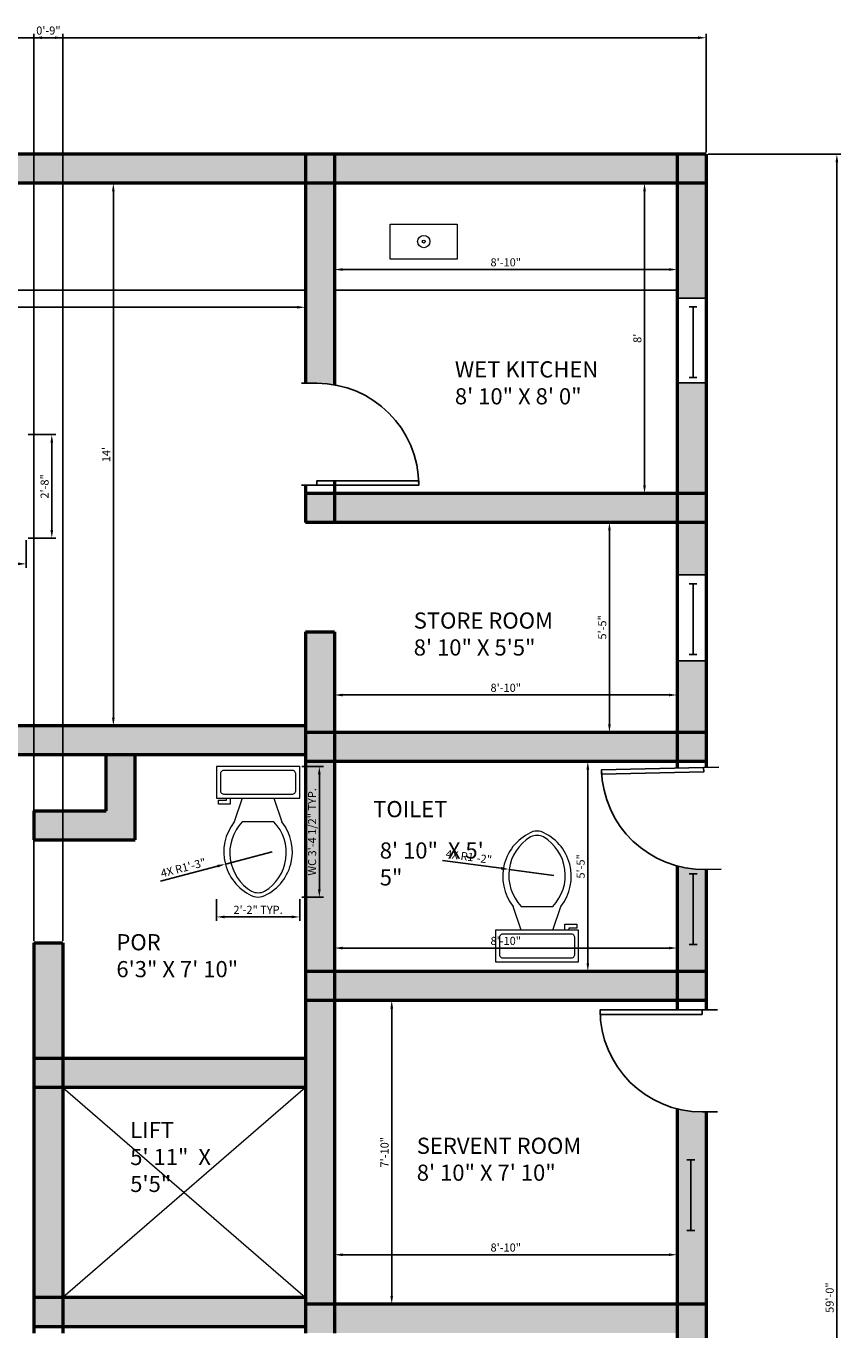
# Model space of a CAD drawing. Units: millimetres. Extents: x 2481 to 3088, y 720 to 1513.
# Tile 4 of 4: x 2836 to 3088, y 1109 to 1513. Entities that reach past the tile are written whole.
import ezdxf

# ---------------------------------------------------------------- set-up
doc = ezdxf.new("R2010")
doc.units = ezdxf.units.MM
for name, color, linetype, lineweight in [('A-FLOR-CASE', 150, 'Continuous', 25), ('A-FLOR-EVTR', 150, 'Continuous', 18), ('A-FLOR-FIXT', 2, 'Continuous', 18), ('A-WALL-PATT', 5, 'Continuous', 13), ('DIMENSIONS', 10, 'Continuous', 18), ('DOORS', 213, 'Continuous', 25), ('TEXT', 80, 'Continuous', 25), ('WALLS', 150, 'Continuous', 50), ('WINDOWS', 23, 'Continuous', 25)]:
    doc.layers.add(name, color=color, linetype=linetype, lineweight=lineweight)
doc.styles.get("Standard").update_dxf_attribs({"font": 'arial.ttf'})
doc.dimstyles.new('ISO-25', dxfattribs={"dimtxt": 2.5, "dimasz": 2.5, "dimexe": 1.25, "dimexo": 0.625, "dimtad": 1, "dimdec": 0, "dimlunit": 3, "dimtxsty": 'Standard', "dimcen": 2.5, "dimadec": 0, "dimazin": 0, "dimtfac": 1, "dimtdec": 0, "dimtmove": 0, "dimatfit": 3, "dimfxl": 1, "dimarcsym": 0})

# ---------------------------------------------------------------- blocks, each defined once
blk = doc.blocks.new('*U2')
for p, q in [((0, 0), (0, -6)), ((40, 0), (40, -6))]:
    blk.add_line(p, q)
blk.add_lwpolyline([(0, 0), (0, 40), (1.75, 40), (1.75, 0)], close=True)
blk.add_arc((0, 0), 40, 0, 90)
blk = doc.blocks.new('*U6')
for p, q in [((0, 4), (0, 0)), ((0, 2), (36, 2)), ((36, 4), (36, 0))]:
    blk.add_line(p, q)
blk = doc.blocks.new('Toilet - top')
for p, q in [((9.5, -6), (9.5, -2)), ((-10, -8.5), (-8, -8.5)), ((-10, -9.5), (-10, -8.5)), ((-7, -9.5), (-10, -9.5)), ((-8, -8.5), (-8, -8)), ((-7, -8), (-7, -9.5)), ((-4, -8), (-6, -14)), ((4, -8), (6, -14)), ((4, -14), (-4, -14))]:
    blk.add_line(p, q)
blk.add_lwpolyline([(10.5, -8), (10.5, 0), (-10.5, 0), (-10.5, -8)], close=True)
for points in [[(-9.5, -2), (-9.5, -6)], [(8.5, -1), (-8.5, -1)], [(-8.5, -7), (8.5, -7)]]:
    blk.add_lwpolyline(points)
for centre, radius, start, end in [((-8.62, -1.88), 0.884, 81.8699, 188.1301), ((8.62, -1.88), 0.884, 351.8699, 98.1301), ((-8.62, -6.12), 0.884, 171.8699, 278.1301), ((8.62, -6.12), 0.884, 261.8699, 8.1301), ((3.52, -21.58), 12.17, 141.4691, 247.9714), ((4.2, -21.82), 11.33, 136.3677, 238.9468), ((-3.52, -21.58), 12.17, 292.0284, 38.5307), ((-4.2, -21.82), 11.33, 301.053, 43.6321), ((0, -27.88), 4, 245.7318, 294.2682), ((0, -29), 4, 254.8605, 285.1395)]:
    blk.add_arc(centre, radius, start, end)
blk = doc.blocks.new('*D15')
at = {"layer": 'Defpoints', "color": 0, "transparency": 16777216}
for p in [(2857.65, 1464.49), (2857.65, 1296.49), (2863.09, 1296.49)]:
    blk.add_point(p, dxfattribs=at)
at = {"layer": 'DIMENSIONS', "color": 0, "lineweight": -2, "transparency": 16777216}
for p, q in [((2858.27, 1464.49), (2864.34, 1464.49)), ((2863.09, 1461.99), (2863.09, 1298.99)), ((2858.27, 1296.49), (2864.34, 1296.49))]:
    blk.add_line(p, q, dxfattribs=at)
at = {"layer": 'DIMENSIONS', "color": 0, "transparency": 16777216}
for points in [[(2862.68, 1461.99), (2863.51, 1461.99), (2863.09, 1464.49)], [(2862.68, 1298.99), (2863.51, 1298.99), (2863.09, 1296.49)]]:
    blk.add_solid(points, dxfattribs=at)
at = {"layer": 'DIMENSIONS', "color": 0, "transparency": 16777216, "insert": (2861.21, 1380.49), "char_height": 2.5, "attachment_point": 5, "rotation": 90}
blk.add_mtext("14'", dxfattribs=at)
blk = doc.blocks.new('*D16')
at = {"layer": 'Defpoints', "color": 0, "transparency": 16777216}
for p in [(2599.5, 1428.42), (2922.5, 1426.09), (2922.5, 1426.09)]:
    blk.add_point(p, dxfattribs=at)
at = {"layer": 'DIMENSIONS', "color": 0, "lineweight": -2, "transparency": 16777216}
for p, q in [((2599.5, 1427.79), (2599.5, 1424.84)), ((2602, 1426.09), (2920, 1426.09)), ((2922.5, 1426.72), (2922.5, 1427.34))]:
    blk.add_line(p, q, dxfattribs=at)
at = {"layer": 'DIMENSIONS', "color": 0, "transparency": 16777216}
for points in [[(2602, 1426.51), (2602, 1425.68), (2599.5, 1426.09)], [(2920, 1426.51), (2920, 1425.68), (2922.5, 1426.09)]]:
    blk.add_solid(points, dxfattribs=at)
at = {"layer": 'DIMENSIONS', "color": 0, "transparency": 16777216, "insert": (2761, 1428), "char_height": 2.5, "attachment_point": 5}
blk.add_mtext('26\'-11"', dxfattribs=at)
blk = doc.blocks.new('*D17')
at = {"layer": 'Defpoints', "color": 0, "transparency": 16777216}
for p in [(3031.12, 1464.49), (3027.44, 1368.49), (3031.12, 1368.49)]:
    blk.add_point(p, dxfattribs=at)
at = {"layer": 'DIMENSIONS', "color": 0, "lineweight": -2, "transparency": 16777216}
for p, q in [((3030.49, 1464.49), (3026.19, 1464.49)), ((3027.44, 1461.99), (3027.44, 1370.99)), ((3030.49, 1368.49), (3026.19, 1368.49))]:
    blk.add_line(p, q, dxfattribs=at)
at = {"layer": 'DIMENSIONS', "color": 0, "transparency": 16777216}
for points in [[(3027.02, 1461.99), (3027.86, 1461.99), (3027.44, 1464.49)], [(3027.02, 1370.99), (3027.86, 1370.99), (3027.44, 1368.49)]]:
    blk.add_solid(points, dxfattribs=at)
at = {"layer": 'DIMENSIONS', "color": 0, "transparency": 16777216, "insert": (3025.54, 1416.49), "char_height": 2.5, "attachment_point": 5, "rotation": 90}
blk.add_mtext("8'", dxfattribs=at)
blk = doc.blocks.new('*D18')
at = {"layer": 'Defpoints', "color": 0, "transparency": 16777216}
for p in [(2931.5, 1440.32), (2931.5, 1437.78), (3037.5, 1440.32)]:
    blk.add_point(p, dxfattribs=at)
at = {"layer": 'DIMENSIONS', "color": 0, "lineweight": -2, "transparency": 16777216}
for p, q in [((2931.5, 1439.69), (2931.5, 1436.53)), ((3035, 1437.78), (2934, 1437.78)), ((3037.5, 1439.69), (3037.5, 1436.53))]:
    blk.add_line(p, q, dxfattribs=at)
at = {"layer": 'DIMENSIONS', "color": 0, "transparency": 16777216}
for points in [[(2934, 1438.2), (2934, 1437.37), (2931.5, 1437.78)], [(3035, 1438.2), (3035, 1437.37), (3037.5, 1437.78)]]:
    blk.add_solid(points, dxfattribs=at)
at = {"layer": 'DIMENSIONS', "color": 0, "transparency": 16777216, "insert": (2984.5, 1439.69), "char_height": 2.5, "attachment_point": 5}
blk.add_mtext('8\'-10"', dxfattribs=at)
blk = doc.blocks.new('*D19')
at = {"layer": 'Defpoints', "color": 0, "transparency": 16777216}
for p in [(3016.58, 1359.49), (3016.58, 1294.49), (3016.58, 1294.49)]:
    blk.add_point(p, dxfattribs=at)
at = {"layer": 'DIMENSIONS', "color": 0, "lineweight": -2, "transparency": 16777216}
for p, q in [((3016.58, 1356.99), (3016.58, 1296.99)), ((3017.21, 1359.49), (3017.83, 1359.49)), ((3017.21, 1294.49), (3017.83, 1294.49))]:
    blk.add_line(p, q, dxfattribs=at)
at = {"layer": 'DIMENSIONS', "color": 0, "transparency": 16777216}
for points in [[(3016.17, 1356.99), (3017, 1356.99), (3016.58, 1359.49)], [(3016.17, 1296.99), (3017, 1296.99), (3016.58, 1294.49)]]:
    blk.add_solid(points, dxfattribs=at)
at = {"layer": 'DIMENSIONS', "color": 0, "transparency": 16777216, "insert": (3014.69, 1326.99), "char_height": 2.5, "attachment_point": 5, "rotation": 90}
blk.add_mtext('5\'-5"', dxfattribs=at)
blk = doc.blocks.new('*D20')
at = {"layer": 'Defpoints', "color": 0, "transparency": 16777216}
for p in [(2931.5, 1306.06), (2931.5, 1306.06), (3037.5, 1306.06)]:
    blk.add_point(p, dxfattribs=at)
at = {"layer": 'DIMENSIONS', "color": 0, "lineweight": -2, "transparency": 16777216}
for p, q in [((2931.5, 1306.68), (2931.5, 1307.31)), ((3035, 1306.06), (2934, 1306.06)), ((3037.5, 1306.68), (3037.5, 1307.31))]:
    blk.add_line(p, q, dxfattribs=at)
at = {"layer": 'DIMENSIONS', "color": 0, "transparency": 16777216}
for points in [[(2934, 1306.47), (2934, 1305.64), (2931.5, 1306.06)], [(3035, 1306.47), (3035, 1305.64), (3037.5, 1306.06)]]:
    blk.add_solid(points, dxfattribs=at)
at = {"layer": 'DIMENSIONS', "color": 0, "transparency": 16777216, "insert": (2984.5, 1307.96), "char_height": 2.5, "attachment_point": 5}
blk.add_mtext('8\'-10"', dxfattribs=at)
blk = doc.blocks.new('*D21')
at = {"layer": 'Defpoints', "color": 0, "transparency": 16777216}
for p in [(2931.5, 1132.77), (2931.5, 1132.77), (3037.5, 1132.77)]:
    blk.add_point(p, dxfattribs=at)
at = {"layer": 'DIMENSIONS', "color": 0, "lineweight": -2, "transparency": 16777216}
for p, q in [((2931.5, 1133.39), (2931.5, 1134.02)), ((3035, 1132.77), (2934, 1132.77)), ((3037.5, 1133.39), (3037.5, 1134.02))]:
    blk.add_line(p, q, dxfattribs=at)
at = {"layer": 'DIMENSIONS', "color": 0, "transparency": 16777216}
for points in [[(2934, 1133.18), (2934, 1132.35), (2931.5, 1132.77)], [(3035, 1133.18), (3035, 1132.35), (3037.5, 1132.77)]]:
    blk.add_solid(points, dxfattribs=at)
at = {"layer": 'DIMENSIONS', "color": 0, "transparency": 16777216, "insert": (2984.5, 1134.67), "char_height": 2.5, "attachment_point": 5}
blk.add_mtext('8\'-10"', dxfattribs=at)
blk = doc.blocks.new('*D22')
at = {"layer": 'Defpoints', "color": 0, "transparency": 16777216}
for p in [(2947.9, 1211.49), (2947.9, 1117.49), (2949.22, 1117.49)]:
    blk.add_point(p, dxfattribs=at)
at = {"layer": 'DIMENSIONS', "color": 0, "lineweight": -2, "transparency": 16777216}
for p, q in [((2948.52, 1211.49), (2950.47, 1211.49)), ((2949.22, 1208.99), (2949.22, 1119.99)), ((2948.52, 1117.49), (2950.47, 1117.49))]:
    blk.add_line(p, q, dxfattribs=at)
at = {"layer": 'DIMENSIONS', "color": 0, "transparency": 16777216}
for points in [[(2948.81, 1208.99), (2949.64, 1208.99), (2949.22, 1211.49)], [(2948.81, 1119.99), (2949.64, 1119.99), (2949.22, 1117.49)]]:
    blk.add_solid(points, dxfattribs=at)
at = {"layer": 'DIMENSIONS', "color": 0, "transparency": 16777216, "insert": (2947.32, 1164.49), "char_height": 2.5, "attachment_point": 5, "rotation": 90}
blk.add_mtext('7\'-10"', dxfattribs=at)
blk = doc.blocks.new('*D23')
at = {"layer": 'Defpoints', "color": 0, "transparency": 16777216}
for p in [(3009.89, 1285.49), (3009.89, 1220.49), (3009.89, 1220.49)]:
    blk.add_point(p, dxfattribs=at)
at = {"layer": 'DIMENSIONS', "color": 0, "lineweight": -2, "transparency": 16777216}
for p, q in [((3010.52, 1285.49), (3011.14, 1285.49)), ((3009.89, 1282.99), (3009.89, 1222.99)), ((3010.52, 1220.49), (3011.14, 1220.49))]:
    blk.add_line(p, q, dxfattribs=at)
at = {"layer": 'DIMENSIONS', "color": 0, "transparency": 16777216}
for points in [[(3009.48, 1282.99), (3010.31, 1282.99), (3009.89, 1285.49)], [(3009.48, 1222.99), (3010.31, 1222.99), (3009.89, 1220.49)]]:
    blk.add_solid(points, dxfattribs=at)
at = {"layer": 'DIMENSIONS', "color": 0, "transparency": 16777216, "insert": (3008, 1252.99), "char_height": 2.5, "attachment_point": 5, "rotation": 90}
blk.add_mtext('5\'-5"', dxfattribs=at)
blk = doc.blocks.new('*D24')
at = {"layer": 'Defpoints', "color": 0, "transparency": 16777216}
for p in [(2931.5, 1234.16), (3037.5, 1232.04), (3037.5, 1227.71)]:
    blk.add_point(p, dxfattribs=at)
at = {"layer": 'DIMENSIONS', "color": 0, "lineweight": -2, "transparency": 16777216}
for p, q in [((2931.5, 1233.54), (2931.5, 1226.46)), ((3037.5, 1231.41), (3037.5, 1226.46)), ((2934, 1227.71), (3035, 1227.71))]:
    blk.add_line(p, q, dxfattribs=at)
at = {"layer": 'DIMENSIONS', "color": 0, "transparency": 16777216}
for points in [[(2934, 1228.13), (2934, 1227.29), (2931.5, 1227.71)], [(3035, 1228.13), (3035, 1227.29), (3037.5, 1227.71)]]:
    blk.add_solid(points, dxfattribs=at)
at = {"layer": 'DIMENSIONS', "color": 0, "transparency": 16777216, "insert": (2984.5, 1229.61), "char_height": 2.5, "attachment_point": 5}
blk.add_mtext('8\'-10"', dxfattribs=at)
blk = doc.blocks.new('*D31')
at = {"layer": 'Defpoints', "color": 0, "transparency": 16777216}
for p in [(2920.75, 1283.95), (2926.83, 1283.95), (2920.75, 1243.43)]:
    blk.add_point(p, dxfattribs=at)
at = {"layer": 'DIMENSIONS', "color": 0, "lineweight": -2, "transparency": 16777216}
for p, q in [((2921.37, 1283.95), (2928.08, 1283.95)), ((2926.83, 1245.93), (2926.83, 1281.45)), ((2921.37, 1243.43), (2928.08, 1243.43))]:
    blk.add_line(p, q, dxfattribs=at)
at = {"layer": 'DIMENSIONS', "color": 0, "transparency": 16777216}
for points in [[(2926.41, 1281.45), (2927.24, 1281.45), (2926.83, 1283.95)], [(2926.41, 1245.93), (2927.24, 1245.93), (2926.83, 1243.43)]]:
    blk.add_solid(points, dxfattribs=at)
at = {"layer": 'DIMENSIONS', "color": 0, "transparency": 16777216, "insert": (2924.91, 1263.69), "char_height": 2.5, "attachment_point": 5, "rotation": 90}
blk.add_mtext('WC 3\'-4 1/2" TYP.', dxfattribs=at)
blk = doc.blocks.new('*D32')
at = {"layer": 'Defpoints', "color": 0, "transparency": 16777216}
for p in [(2894.99, 1243.43), (2920.75, 1243.43), (2920.75, 1237.35)]:
    blk.add_point(p, dxfattribs=at)
at = {"layer": 'DIMENSIONS', "color": 0, "lineweight": -2, "transparency": 16777216}
for p, q in [((2894.99, 1242.8), (2894.99, 1236.1)), ((2920.75, 1242.8), (2920.75, 1236.1)), ((2897.49, 1237.35), (2918.25, 1237.35))]:
    blk.add_line(p, q, dxfattribs=at)
at = {"layer": 'DIMENSIONS', "color": 0, "transparency": 16777216}
for points in [[(2897.49, 1237.77), (2897.49, 1236.93), (2894.99, 1237.35)], [(2918.25, 1237.77), (2918.25, 1236.93), (2920.75, 1237.35)]]:
    blk.add_solid(points, dxfattribs=at)
at = {"layer": 'DIMENSIONS', "color": 0, "transparency": 16777216, "insert": (2907.87, 1239.23), "char_height": 2.5, "attachment_point": 5}
blk.add_mtext('2\'-2" TYP.', dxfattribs=at)
blk = doc.blocks.new('*D33')
at = {"layer": 'Defpoints', "color": 0, "transparency": 16777216}
for p in [(2783.07, 1354.61), (2836.1, 1354.61), (2836.1, 1346.66)]:
    blk.add_point(p, dxfattribs=at)
at = {"layer": 'DIMENSIONS', "color": 0, "lineweight": -2, "transparency": 16777216}
for p, q in [((2783.07, 1353.98), (2783.07, 1345.41)), ((2836.1, 1353.98), (2836.1, 1345.41)), ((2785.57, 1346.66), (2833.6, 1346.66))]:
    blk.add_line(p, q, dxfattribs=at)
at = {"layer": 'DIMENSIONS', "color": 0, "transparency": 16777216}
for points in [[(2785.57, 1347.07), (2785.57, 1346.24), (2783.07, 1346.66)], [(2833.6, 1347.07), (2833.6, 1346.24), (2836.1, 1346.66)]]:
    blk.add_solid(points, dxfattribs=at)
at = {"layer": 'DIMENSIONS', "color": 0, "transparency": 16777216, "insert": (2809.58, 1348.57), "char_height": 2.5, "attachment_point": 5}
blk.add_mtext('DINING SET 4\'-5"', dxfattribs=at)
blk = doc.blocks.new('*D34')
at = {"layer": 'Defpoints', "color": 0, "transparency": 16777216}
for p in [(2836.1, 1386.66), (2844.05, 1386.66), (2836.1, 1354.61)]:
    blk.add_point(p, dxfattribs=at)
at = {"layer": 'DIMENSIONS', "color": 0, "lineweight": -2, "transparency": 16777216}
for p, q in [((2836.72, 1386.66), (2845.3, 1386.66)), ((2844.05, 1357.11), (2844.05, 1384.16)), ((2836.72, 1354.61), (2845.3, 1354.61))]:
    blk.add_line(p, q, dxfattribs=at)
at = {"layer": 'DIMENSIONS', "color": 0, "transparency": 16777216}
for points in [[(2843.63, 1384.16), (2844.47, 1384.16), (2844.05, 1386.66)], [(2843.63, 1357.11), (2844.47, 1357.11), (2844.05, 1354.61)]]:
    blk.add_solid(points, dxfattribs=at)
at = {"layer": 'DIMENSIONS', "color": 0, "transparency": 16777216, "insert": (2842.15, 1370.63), "char_height": 2.5, "attachment_point": 5, "rotation": 90}
blk.add_mtext('2\'-8"', dxfattribs=at)
blk = doc.blocks.new('*D38')
at = {"layer": 'Defpoints', "color": 0, "transparency": 16777216}
for p in [(3046.5, 1473.49), (3086.95, 1473.49), (3046.5, 765.49)]:
    blk.add_point(p, dxfattribs=at)
at = {"layer": 'DIMENSIONS', "color": 0, "lineweight": -2, "transparency": 16777216}
for p, q in [((3047.12, 1473.49), (3088.2, 1473.49)), ((3086.95, 767.99), (3086.95, 1470.99)), ((3047.12, 765.49), (3088.2, 765.49))]:
    blk.add_line(p, q, dxfattribs=at)
at = {"layer": 'DIMENSIONS', "color": 0, "transparency": 16777216}
for points in [[(3086.53, 1470.99), (3087.36, 1470.99), (3086.95, 1473.49)], [(3086.53, 767.99), (3087.36, 767.99), (3086.95, 765.49)]]:
    blk.add_solid(points, dxfattribs=at)
at = {"layer": 'DIMENSIONS', "color": 0, "transparency": 16777216, "insert": (3085.04, 1119.49), "char_height": 2.5, "attachment_point": 5, "rotation": 90}
blk.add_mtext('59\'-0"', dxfattribs=at)
blk = doc.blocks.new('*D39')
at = {"layer": 'Defpoints', "color": 0, "transparency": 16777216}
for p in [(3046.5, 1509.55), (2590.5, 1473.49), (3046.5, 1473.49)]:
    blk.add_point(p, dxfattribs=at)
at = {"layer": 'DIMENSIONS', "color": 0, "lineweight": -2, "transparency": 16777216}
for p, q in [((2590.5, 1474.11), (2590.5, 1510.8)), ((3046.5, 1474.11), (3046.5, 1510.8)), ((2593, 1509.55), (3044, 1509.55))]:
    blk.add_line(p, q, dxfattribs=at)
at = {"layer": 'DIMENSIONS', "color": 0, "transparency": 16777216}
for points in [[(2593, 1509.97), (2593, 1509.13), (2590.5, 1509.55)], [(3044, 1509.97), (3044, 1509.13), (3046.5, 1509.55)]]:
    blk.add_solid(points, dxfattribs=at)
at = {"layer": 'DIMENSIONS', "color": 0, "transparency": 16777216, "insert": (2818.5, 1511.45), "char_height": 2.5, "attachment_point": 5}
blk.add_mtext('38\'-0"', dxfattribs=at)
blk = doc.blocks.new('*D41')
at = {"layer": 'Defpoints', "color": 0, "transparency": 16777216}
for p in [(2847.5, 1509.55), (2838.5, 1229.29), (2847.5, 1229.29)]:
    blk.add_point(p, dxfattribs=at)
at = {"layer": 'DIMENSIONS', "color": 0, "lineweight": -2, "transparency": 16777216}
for p, q in [((2838.5, 1229.91), (2838.5, 1510.8)), ((2847.5, 1229.91), (2847.5, 1510.8)), ((2841, 1509.55), (2845, 1509.55))]:
    blk.add_line(p, q, dxfattribs=at)
at = {"layer": 'DIMENSIONS', "color": 0, "transparency": 16777216}
for points in [[(2841, 1509.97), (2841, 1509.13), (2838.5, 1509.55)], [(2845, 1509.97), (2845, 1509.13), (2847.5, 1509.55)]]:
    blk.add_solid(points, dxfattribs=at)
at = {"layer": 'DIMENSIONS', "color": 0, "transparency": 16777216, "insert": (2843, 1511.45), "char_height": 2.5, "attachment_point": 5}
blk.add_mtext('0\'-9"', dxfattribs=at)
blk = doc.blocks.new('*D50')
at = {"layer": 'Defpoints', "color": 0, "transparency": 16777216}
for p in [(2912.19, 1257.49), (2897.75, 1253.7)]:
    blk.add_point(p, dxfattribs=at)
at = {"layer": 'DIMENSIONS', "color": 0, "lineweight": -2, "transparency": 16777216}
for p, q in [((2912.19, 1257.49), (2897.75, 1253.7)), ((2877.67, 1248.42), (2895.34, 1253.06))]:
    blk.add_line(p, q, dxfattribs=at)
at = {"layer": 'DIMENSIONS', "color": 0, "transparency": 16777216}
blk.add_solid([(2895.23, 1253.46), (2895.44, 1252.66), (2897.75, 1253.7)], dxfattribs=at)
at = {"layer": 'DIMENSIONS', "color": 0, "transparency": 16777216, "insert": (2884.81, 1252.26), "char_height": 2.5, "attachment_point": 5, "rotation": 14.7187}
blk.add_mtext('4X R1\'-3"', dxfattribs=at)
blk = doc.blocks.new('*D51')
at = {"layer": 'Defpoints', "color": 0, "transparency": 16777216}
for p in [(2985.56, 1252.06), (2999.33, 1250.21)]:
    blk.add_point(p, dxfattribs=at)
at = {"layer": 'DIMENSIONS', "color": 0, "lineweight": -2, "transparency": 16777216}
for p, q in [((2964.98, 1254.83), (2983.08, 1252.4)), ((2999.33, 1250.21), (2985.56, 1252.06))]:
    blk.add_line(p, q, dxfattribs=at)
at = {"layer": 'DIMENSIONS', "color": 0, "transparency": 16777216}
blk.add_solid([(2983.13, 1252.81), (2983.02, 1251.98), (2985.56, 1252.06)], dxfattribs=at)
at = {"layer": 'DIMENSIONS', "color": 0, "transparency": 16777216, "insert": (2973.04, 1255.64), "char_height": 2.5, "attachment_point": 5, "rotation": 352.3363}
blk.add_mtext('4X R1\'-2"', dxfattribs=at)

msp = doc.modelspace()

# ---------------------------------------------------------------- hatches: boundary and pattern name
at = {"layer": 'A-WALL-PATT'}
h = msp.add_hatch(color=256, dxfattribs=at)
h.dxf.hatch_style = 1
h.paths.add_polyline_path([(2599.5, 1473.49), (2590.5, 1473.49), (2590.5, 1464.49), (2599.5, 1464.49)])
h.paths.add_polyline_path([(2599.5, 1464.49), (2590.5, 1464.49), (2590.5, 1447.8), (2599.5, 1447.8)])
h.paths.add_polyline_path([(2625.38, 1473.49), (2599.5, 1473.49), (2599.5, 1464.49), (2625.38, 1464.49)])
h.paths.add_polyline_path([(2805.36, 1473.49), (2710.95, 1473.49), (2710.95, 1464.49), (2805.36, 1464.49)])
h.paths.add_polyline_path([(2922.5, 1473.49), (2830.18, 1473.49), (2830.18, 1464.49), (2922.5, 1464.49)])
h.paths.add_polyline_path([(2931.5, 1473.49), (2922.5, 1473.49), (2922.5, 1464.49), (2931.5, 1464.49)])
h.paths.add_polyline_path([(2931.5, 1464.49), (2922.5, 1464.49), (2922.5, 1402.56), (2926.01, 1402.56, -0.043673), (2931.5, 1402.08)])
h.paths.add_polyline_path([(2931.5, 1368.49), (2922.5, 1368.49), (2922.5, 1359.49), (2931.5, 1359.49)])
h.paths.add_polyline_path([(2922.5, 1296.49), (2675.15, 1296.49), (2675.15, 1287.49), (2922.5, 1287.49)])
h.paths.add_polyline_path([(2931.5, 1294.49), (2922.5, 1294.49), (2922.5, 1287.49), (2922.5, 1285.49), (2931.5, 1285.49)])
h.paths.add_polyline_path([(3037.5, 1294.49), (2931.5, 1294.49), (2931.5, 1285.49), (3037.5, 1285.49)])
h.paths.add_polyline_path([(3046.5, 1294.49), (3037.5, 1294.49), (3037.5, 1285.49), (3046.5, 1285.49)])
h.paths.add_polyline_path([(3046.5, 1316.66), (3037.5, 1316.66), (3037.5, 1294.49), (3046.5, 1294.49)])
h.paths.add_polyline_path([(3046.5, 1359.49), (3037.5, 1359.49), (3037.5, 1343.26), (3046.5, 1343.26)])
h.paths.add_polyline_path([(3046.5, 1368.49), (3037.5, 1368.49), (3037.5, 1359.49), (3046.5, 1359.49)])
h.paths.add_polyline_path([(3037.5, 1368.49), (2931.5, 1368.49), (2931.5, 1359.49), (3037.5, 1359.49)])
h.paths.add_polyline_path([(2599.5, 1361.25), (2590.5, 1361.25), (2590.5, 1233.6), (2599.5, 1233.6)])
h.paths.add_polyline_path([(2535.5, 1110.49), (2526.5, 1110.49), (2526.5, 933.49), (2535.5, 933.49)])
h.paths.add_polyline_path([(2535.5, 1119.49), (2526.5, 1119.49), (2526.5, 1110.49), (2535.5, 1110.49)])
h.paths.add_polyline_path([(2590.5, 1119.49), (2535.5, 1119.49), (2535.5, 1110.49), (2590.5, 1110.49)])
h.paths.add_polyline_path([(2599.5, 1119.49), (2594.5, 1119.49), (2590.5, 1119.49), (2590.5, 1110.49), (2594.5, 1110.49), (2599.5, 1110.49)])
h.paths.add_polyline_path([(2599.5, 1148.41), (2590.5, 1148.41), (2590.5, 1119.49), (2594.5, 1119.49), (2599.5, 1119.49)])
h.paths.add_polyline_path([(2770.14, 1119.49), (2599.5, 1119.49), (2599.5, 1110.49), (2770.14, 1110.49)])
h.paths.add_polyline_path([(3037.5, 1473.49), (2931.5, 1473.49), (2931.5, 1464.49), (3037.5, 1464.49)])
h.paths.add_polyline_path([(3046.5, 1473.49), (3037.5, 1473.49), (3037.5, 1464.49), (3046.5, 1464.49)])
h.paths.add_polyline_path([(2535.5, 842.83), (2535.5, 924.49), (2526.5, 924.49), (2526.5, 774.49), (2535.5, 774.49)])
h.paths.add_polyline_path([(2535.5, 774.49), (2526.5, 774.49), (2526.5, 765.49), (2535.5, 765.49)])
h.paths.add_polyline_path([(3037.5, 774.49), (2945.5, 774.49), (2852.34, 774.49), (2852.34, 765.49), (3037.5, 765.49)])
h.paths.add_polyline_path([(3046.5, 774.49), (3037.5, 774.49), (3037.5, 765.49), (3046.5, 765.49)])
h.paths.add_polyline_path([(3046.5, 882.49), (3037.5, 882.49), (3037.5, 774.49), (3046.5, 774.49)])
h.paths.add_polyline_path([(2768.5, 774.49), (2759.5, 774.49), (2759.5, 765.49), (2768.5, 765.49)])
h.paths.add_polyline_path([(2759.5, 774.49), (2535.5, 774.49), (2535.5, 765.49), (2759.5, 765.49)])
h.paths.add_polyline_path([(2768.5, 781.94), (2759.5, 781.94), (2759.5, 774.49), (2768.5, 774.49)])
h.paths.add_polyline_path([(2768.5, 1015.49), (2759.5, 1015.49), (2759.5, 933.49), (2768.5, 933.49)])
h.paths.add_polyline_path([(2768.5, 933.49), (2759.5, 933.49), (2759.5, 924.49), (2768.5, 924.49)])
h.paths.add_polyline_path([(2768.5, 924.49), (2759.5, 924.49), (2759.5, 864.16), (2768.5, 864.16)])
h.paths.add_polyline_path([(2759.5, 933.49), (2734.57, 933.49), (2734.57, 924.49), (2759.5, 924.49)])
h.paths.add_polyline_path([(2954.5, 1015.49), (2945.5, 1015.49), (2945.5, 842.83), (2954.5, 842.83)])
h.paths.add_polyline_path([(2954.5, 1024.49), (2945.5, 1024.49), (2945.5, 1015.49), (2954.5, 1015.49)])
h.paths.add_polyline_path([(2945.5, 1024.49), (2808.62, 1024.49), (2808.62, 1022.52, -0.056199), (2807.82, 1015.49), (2945.5, 1015.49)])
h.paths.add_polyline_path([(3037.5, 1024.49), (2954.5, 1024.49), (2954.5, 1015.49), (3037.5, 1015.49)])
h.paths.add_polyline_path([(3046.5, 1024.49), (3037.5, 1024.49), (3037.5, 1015.49), (3046.5, 1015.49)])
h.paths.add_polyline_path([(3046.5, 1015.49), (3037.5, 1015.49), (3037.5, 994.13), (3046.5, 994.13)])
h.paths.add_polyline_path([(3046.5, 928.1), (3037.5, 928.1), (3037.5, 891.49), (3046.5, 891.49)])
h.paths.add_polyline_path([(3046.5, 891.49), (3037.5, 891.49), (3037.5, 882.49), (3046.5, 882.49)])
h.paths.add_polyline_path([(3037.5, 891.49), (2987.62, 891.49), (2987.62, 882.49), (3037.5, 882.49)])
h.paths.add_polyline_path([(2768.5, 1024.49), (2759.5, 1024.49), (2759.5, 1015.49), (2768.5, 1015.49)])
h.paths.add_polyline_path([(2777.03, 1022.52), (2777.03, 1024.49), (2768.5, 1024.49), (2768.5, 1015.49), (2777.03, 1015.49)])
h = msp.add_hatch(color=256, dxfattribs=at)
h.dxf.hatch_style = 1
h.paths.add_polyline_path([(3046.5, 1464.49), (3037.5, 1464.49), (3037.5, 1428.96), (3046.5, 1428.96)])
h.paths.add_polyline_path([(3046.5, 1402.75), (3037.5, 1402.75), (3037.5, 1368.49), (3046.5, 1368.49)])
h = msp.add_hatch(color=256, dxfattribs=at)
h.dxf.hatch_style = 1
h.paths.add_polyline_path([(2931.5, 1211.49), (2922.5, 1211.49), (2922.5, 1117.49), (2931.5, 1117.49)])
h.paths.add_polyline_path([(2931.5, 1285.49), (2922.5, 1285.49), (2922.5, 1220.49), (2931.5, 1220.49)])
h.paths.add_polyline_path([(2931.5, 1325.63), (2922.5, 1325.63), (2922.5, 1294.49), (2931.5, 1294.49)])
h.paths.add_polyline_path([(2869.83, 1270.23), (2869.83, 1287.49), (2860.83, 1287.49), (2860.83, 1270.23), (2838.5, 1270.23), (2838.5, 1261.23), (2860.83, 1261.23), (2869.83, 1261.23)])
h.paths.add_polyline_path([(3037.5, 1220.49), (2931.5, 1220.49), (2931.5, 1211.49), (3037.5, 1211.49)])
h.paths.add_polyline_path([(2931.5, 1220.49), (2922.5, 1220.49), (2922.5, 1211.49), (2931.5, 1211.49)])
h.paths.add_polyline_path([(3046.5, 1220.49), (3037.5, 1220.49), (3037.5, 1211.49), (3046.5, 1211.49)])
h.paths.add_polyline_path([(3046.5, 1252.04), (3046.4, 1252.04, -0.071368), (3037.5, 1253.12), (3037.5, 1220.49), (3046.5, 1220.49)])
h.paths.add_polyline_path([(2847.5, 1193.49), (2838.5, 1193.49), (2838.5, 1184.49), (2847.5, 1184.49)])
h.paths.add_polyline_path([(2922.5, 1193.49), (2847.5, 1193.49), (2847.5, 1184.49), (2922.5, 1184.49)])
h.paths.add_polyline_path([(2847.5, 1229.29), (2838.5, 1229.29), (2838.5, 1193.49), (2847.5, 1193.49)])
h.paths.add_polyline_path([(2847.5, 1184.49), (2838.5, 1184.49), (2838.5, 1119.49), (2847.5, 1119.49)])
h.paths.add_polyline_path([(2922.5, 1119.49), (2847.5, 1119.49), (2847.5, 1110.49), (2922.5, 1110.49)])
h.paths.add_polyline_path([(2847.5, 1119.49), (2838.5, 1119.49), (2838.5, 1110.49), (2847.5, 1110.49)])
h.paths.add_polyline_path([(3037.5, 1117.49), (2931.5, 1117.49), (2931.5, 1108.49), (3037.5, 1108.49)])
h.paths.add_polyline_path([(2931.5, 1117.49), (2922.5, 1117.49), (2922.5, 1110.49), (2922.5, 1108.49), (2931.5, 1108.49)])
h.paths.add_polyline_path([(3046.5, 1117.49), (3037.5, 1117.49), (3037.5, 1108.49), (3046.5, 1108.49)])
h.paths.add_polyline_path([(3046.5, 1176.98), (3045.26, 1176.98, -0.062137), (3037.5, 1177.95), (3037.5, 1117.49), (3046.5, 1117.49)])
h.paths.add_polyline_path([(3046.5, 1108.49), (3037.5, 1108.49), (3037.5, 1101.52), (3046.5, 1101.52)])
h.paths.add_polyline_path([(3046.5, 1024.49), (3037.5, 1024.49), (3037.5, 1015.49), (3046.5, 1015.49)])
h.paths.add_polyline_path([(3046.5, 1036.41), (3037.5, 1036.41), (3037.5, 1024.49), (3046.5, 1024.49)])

# ---------------------------------------------------------------- linework, layer by layer
at = {"layer": 'A-FLOR-CASE'}
for p, q in [((2753.35, 1431.44), (2922.5, 1431.44)), ((2931.5, 1431.44), (3037.5, 1431.44))]:
    msp.add_line(p, q, dxfattribs=at)
at = {"layer": 'A-FLOR-EVTR'}
for p, q in [((2847.5, 1184.49), (2922.5, 1119.49)), ((2922.5, 1184.49), (2847.5, 1119.49)), ((2922.5, 1119.49), (2922.5, 1119.49))]:
    msp.add_line(p, q, dxfattribs=at)
at = {"layer": 'A-FLOR-FIXT'}
msp.add_lwpolyline([(2948.75, 1451.84), (2969.51, 1451.84), (2969.51, 1441.04), (2948.75, 1441.04)], close=True, dxfattribs=at)
for radius in [1.9, 0.467]:
    msp.add_circle((2959.13, 1446.44), radius, dxfattribs=at)
at = {"layer": 'WALLS'}
for p, q in [((3046.5, 1473.49), (2590.5, 1473.49)), ((2922.5, 1473.49), (2922.5, 1402.56)), ((2931.5, 1473.49), (2931.5, 1402.08)), ((3037.5, 1473.49), (3037.5, 1283.44)), ((3046.5, 1473.49), (3046.5, 1283.64)), ((3046.5, 1464.49), (2590.5, 1464.49)), ((2922.5, 1370.98), (2922.5, 1359.49)), ((3046.5, 1368.49), (2922.5, 1368.49)), ((2931.5, 1372.36), (2931.5, 1359.49)), ((3046.5, 1359.49), (2922.5, 1359.49)), ((2922.5, 1325.63), (2931.5, 1325.63)), ((2922.5, 1325.63), (2922.5, 1108.49)), ((2931.5, 1325.63), (2931.5, 1108.49)), ((2922.5, 1296.49), (2675.15, 1296.49)), ((3046.5, 1294.49), (2922.5, 1294.49)), ((2922.5, 1287.49), (2675.15, 1287.49)), ((2860.83, 1270.23), (2860.83, 1287.49)), ((2869.83, 1270.23), (2869.83, 1287.49)), ((3046.5, 1285.49), (2922.5, 1285.49)), ((2838.5, 1270.23), (2860.83, 1270.23)), ((2838.5, 1270.23), (2838.5, 1261.23)), ((2869.83, 1261.23), (2869.83, 1270.23)), ((2838.5, 1261.23), (2860.83, 1261.23)), ((2860.83, 1261.23), (2869.83, 1261.23)), ((3037.5, 1253.12), (3037.5, 1208.56)), ((3046.5, 1252.04), (3046.5, 1208.56)), ((2838.5, 1229.29), (2847.5, 1229.29)), ((2838.5, 1229.29), (2838.5, 1108.49)), ((2847.5, 1229.29), (2847.5, 1108.49)), ((3046.5, 1220.49), (2922.5, 1220.49)), ((3046.5, 1211.49), (2922.5, 1211.49)), ((2922.5, 1193.49), (2838.5, 1193.49)), ((2922.5, 1184.49), (2838.5, 1184.49)), ((3037.5, 1177.95), (3037.5, 765.49)), ((3046.5, 1176.98), (3046.5, 765.49)), ((2922.5, 1119.49), (2838.5, 1119.49)), ((3046.5, 1117.49), (2922.5, 1117.49)), ((2922.5, 1110.49), (2838.5, 1110.49))]:
    msp.add_line(p, q, dxfattribs=at)
at = {"layer": 'WINDOWS'}
for p, q in [((3046.5, 1428.96), (3037.5, 1428.96)), ((3046.5, 1402.75), (3037.5, 1402.75)), ((3046.5, 1343.26), (3037.5, 1343.26)), ((3046.5, 1316.66), (3037.5, 1316.66))]:
    msp.add_line(p, q, dxfattribs=at)

# ---------------------------------------------------------------- block references
at = {"layer": 'A-FLOR-FIXT', "xscale": 1.226376039306893, "yscale": 1.226376039306893, "zscale": 1.226376039306893}
msp.add_blockref('Toilet - top', (2907.87, 1283.95), dxfattribs=at)
at = {"layer": 'A-FLOR-FIXT', "xscale": 1.226376039306893, "yscale": 1.226376039306893, "zscale": 1.226376039306893, "rotation": 180}
msp.add_blockref('Toilet - top', (2994.18, 1223.45), dxfattribs=at)
at = {"layer": 'DOORS', "xscale": -0.7896024204950681, "yscale": 0.7896024204950681, "zscale": 0.7896024204950681}
for p, rotation in [((2926.01, 1370.98), 270), ((3045.71, 1283.62), 91.25314531773839), ((3045.26, 1208.56), 90)]:
    msp.add_blockref('*U2', p, dxfattribs=dict(at, rotation=rotation))
at = {"layer": 'WINDOWS', "xscale": 0.6081270561735437, "yscale": 0.6081270561735437, "zscale": 0.6081270561735437, "rotation": 90}
for p in [(3043.66, 1404.39), (3043.66, 1318.57), (3043.72, 1228.84), (3043.01, 1140.27)]:
    msp.add_blockref('*U6', p, dxfattribs=at)

# ---------------------------------------------------------------- texts
at = {"layer": 'TEXT', "char_height": 5, "attachment_point": 1}
for s, width, insert in [('WET KITCHEN \\P8\' 10" X 8\' 0"', 48.3324, (2968.76, 1409.37)), ('STORE ROOM \\P8\' 10" X 5\'5"', 44.4311, (2956.03, 1331.61)), ('TOILET', 61.2491, (2943.48, 1273.23)), ('8\' 10"  X 5\' 5"', 36.0163, (2945.51, 1260.42)), ('POR \\P6\'3" X 7\' 10"', 53.9256, (2864.03, 1232.02)), ('LIFT \\P5\' 11"  X 5\'5"', 31.9277, (2868.31, 1173.86)), ('SERVENT ROOM \\P8\' 10" X 7\' 10"', 54.8556, (2956.97, 1169))]:
    msp.add_mtext_dynamic_manual_height_columns(s, width=width, gutter_width=12.5, heights=[0], dxfattribs=dict(at, insert=insert))

# ---------------------------------------------------------------- dimensions: what is measured, and where the dimension line sits
at = {"layer": 'DIMENSIONS'}
for base, p1, p2, override, picture, middle in [((3046.5, 1509.55), (2590.5, 1473.49), (3046.5, 1473.49), {"dimdec": 1, "dimlfac": 1, "dimrnd": 0, "dimzin": 1, "dimdsep": 46, "dimlunit": 4, "dimfrac": 2}, '*D39', (2818.5, 1511.45)), ((2847.5, 1509.55), (2838.5, 1229.29), (2847.5, 1229.29), {"dimdec": 1, "dimlfac": 1, "dimrnd": 0, "dimzin": 1, "dimdsep": 46, "dimlunit": 4, "dimfrac": 2}, '*D41', (2843, 1511.45)), ((2931.5, 1437.78), (3037.5, 1440.32), (2931.5, 1440.32), {"dimclrd": 0, "dimclre": 0, "dimclrt": 0}, '*D18', (2984.5, 1439.69)), ((2922.5, 1426.09), (2599.5, 1428.42), (2922.5, 1426.09), {"dimclrd": 0, "dimclre": 0, "dimclrt": 0}, '*D16', (2761, 1428)), ((2931.5, 1306.06), (3037.5, 1306.06), (2931.5, 1306.06), {"dimclrd": 0, "dimclre": 0, "dimclrt": 0}, '*D20', (2984.5, 1307.96)), ((3037.5, 1227.71), (2931.5, 1234.16), (3037.5, 1232.04), {"dimclrd": 0, "dimclre": 0, "dimclrt": 0}, '*D24', (2984.5, 1229.61)), ((2931.5, 1132.77), (3037.5, 1132.77), (2931.5, 1132.77), {"dimclrd": 0, "dimclre": 0, "dimclrt": 0}, '*D21', (2984.5, 1134.67))]:
    dim = msp.add_linear_dim(base=base, p1=p1, p2=p2, dimstyle='ISO-25', override=override, dxfattribs=at)
    dim.commit()
    dim.dimension.update_dxf_attribs({"geometry": picture, "text_midpoint": middle})
for base, p1, p2, override, picture, middle in [((3086.95, 1473.49), (3046.5, 765.49), (3046.5, 1473.49), {"dimdec": 1, "dimlfac": 1, "dimrnd": 0, "dimzin": 1, "dimdsep": 46, "dimlunit": 4, "dimfrac": 2}, '*D38', (3085.04, 1119.49)), ((2863.09, 1296.49), (2857.65, 1464.49), (2857.65, 1296.49), {"dimclrd": 0, "dimclre": 0, "dimclrt": 0}, '*D15', (2861.21, 1380.49)), ((3027.44, 1368.49), (3031.12, 1464.49), (3031.12, 1368.49), {"dimclrd": 0, "dimclre": 0, "dimclrt": 0}, '*D17', (3025.54, 1416.49)), ((2844.0505, 1386.6589), (2836.0965, 1354.6097), (2836.0965, 1386.6589), {"dimdec": 1, "dimlfac": 1, "dimrnd": 0, "dimzin": 1, "dimdsep": 46, "dimlunit": 4, "dimfrac": 2}, '*D34', (2842.1491, 1370.6343)), ((3016.58, 1294.49), (3016.58, 1359.49), (3016.58, 1294.49), {"dimclrd": 0, "dimclre": 0, "dimclrt": 0}, '*D19', (3014.69, 1326.99)), ((3009.89, 1220.49), (3009.89, 1285.49), (3009.89, 1220.49), {"dimclrd": 0, "dimclre": 0, "dimclrt": 0}, '*D23', (3008, 1252.99)), ((2949.22, 1117.49), (2947.9, 1211.49), (2947.9, 1117.49), {"dimclrd": 0, "dimclre": 0, "dimclrt": 0}, '*D22', (2947.32, 1164.49))]:
    dim = msp.add_linear_dim(base=base, p1=p1, p2=p2, angle=90, dimstyle='ISO-25', override=override, dxfattribs=at)
    dim.commit()
    dim.dimension.update_dxf_attribs({"geometry": picture, "text_midpoint": middle})
for base, p1, p2, text, picture, middle in [((2836.1, 1346.66), (2783.07, 1354.61), (2836.1, 1354.61), 'DINING SET <>', '*D33', (2809.58, 1348.57)), ((2920.75, 1237.35), (2894.99, 1243.43), (2920.75, 1243.43), '<> TYP.', '*D32', (2907.87, 1239.23))]:
    dim = msp.add_linear_dim(base=base, p1=p1, p2=p2, text=text, dimstyle='ISO-25', override={"dimdec": 1, "dimlfac": 1, "dimrnd": 0, "dimzin": 1, "dimdsep": 46, "dimlunit": 4, "dimfrac": 2}, dxfattribs=at)
    dim.commit()
    dim.dimension.update_dxf_attribs({"geometry": picture, "text_midpoint": middle})
dim = msp.add_linear_dim(base=(2926.83, 1283.95), p1=(2920.75, 1243.43), p2=(2920.75, 1283.95), angle=90, text='WC <> TYP.', dimstyle='ISO-25', override={"dimdec": 1, "dimlfac": 1, "dimrnd": 0, "dimzin": 1, "dimdsep": 46, "dimlunit": 4, "dimfrac": 2}, dxfattribs=at)
dim.commit()
dim.dimension.update_dxf_attribs({"geometry": '*D31', "text_midpoint": (2924.91, 1263.69)})
for center, mpoint, picture, middle in [((2999.33, 1250.21), (2985.56, 1252.06), '*D51', (2973.04, 1255.64)), ((2912.19, 1257.49), (2897.75, 1253.7), '*D50', (2884.81, 1252.26))]:
    dim = msp.add_radius_dim(center=center, mpoint=mpoint, text='4X <>', dimstyle='ISO-25', override={"dimdec": 1, "dimlfac": 1, "dimrnd": 0, "dimzin": 1, "dimdsep": 46, "dimlunit": 4, "dimfrac": 2}, dxfattribs=at)
    dim.commit()
    dim.dimension.update_dxf_attribs({"geometry": picture, "text_midpoint": middle})

doc.saveas('drawing.dxf')
